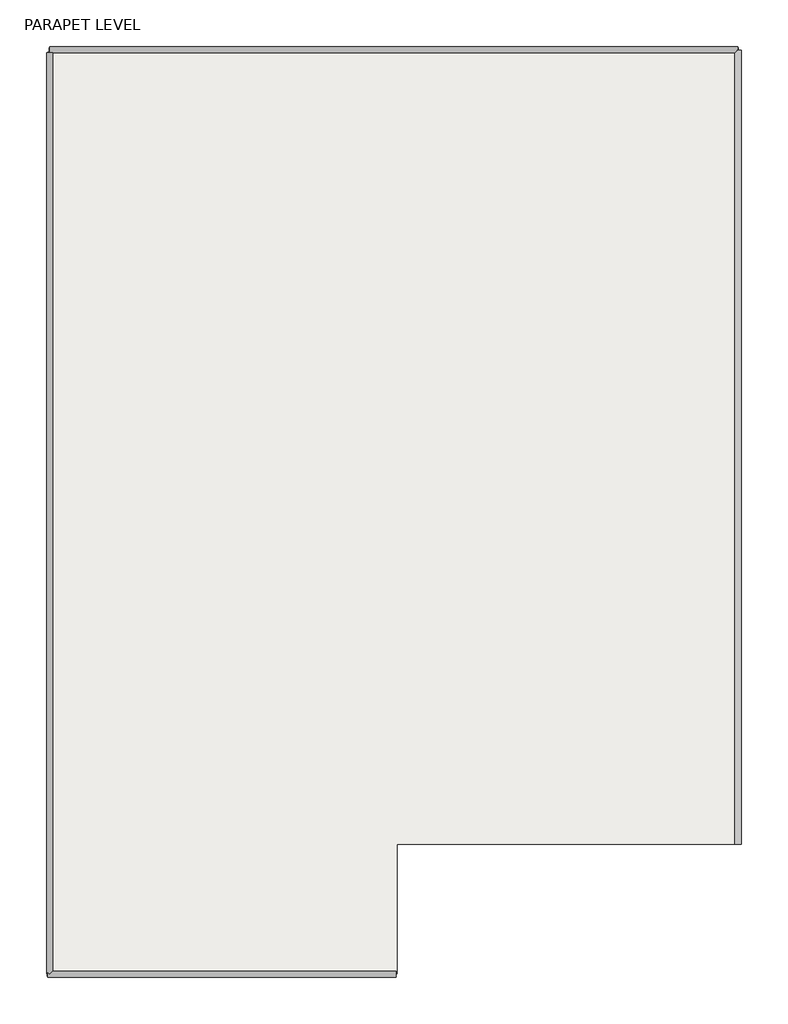
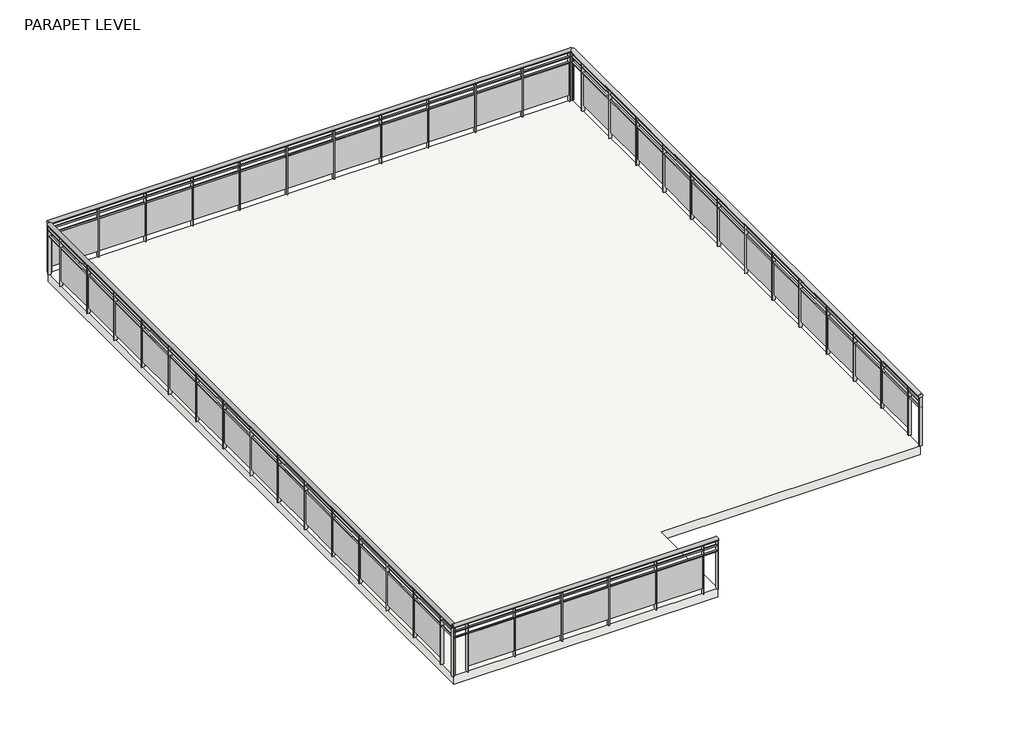
# One storey: 4 railings, 1 slab.
"""IFC4 building model written with IfcOpenShell, lengths in millimetres."""

from ifc_helpers import new_model, si_unit, point, frame, origin, place, context, project, spatial, polyline, ellipse_curve, trimmed, outline, extrude, element, save
from ifc_brep_helpers import plane_surface, extruded_surface, advanced_brep

model = new_model("IFC4")

# Units and contexts
model_context = context("Model", 3, world=origin())
ifc_project = project(units=[si_unit("LENGTHUNIT", "METRE", prefix="MILLI")], contexts=[model_context])

# Site, building, storey
site = spatial("IfcSite", under=ifc_project)
building = spatial("IfcBuilding", under=site)
storey = spatial("IfcBuildingStorey", under=building, Name="PARAPET LEVEL", Elevation=10546.08)

# Railings
placement = place(None, origin())
element("IfcRailing", 1, ObjectType="Glass_Panel-Bottom_Fill", at=placement, inside=storey, context=model_context, shape_type="SolidModel", body=[
    advanced_brep(
    [(-14979.3420435, 42.847874, 10681.6416), (-14979.3420435, -37.152126, 10681.6416), (-6089.3420435, 42.847874, 10681.6416), (-6089.3420435, -37.152126, 10681.6416)],
    [
        (0, 1, ellipse_curve(frame((-14979.3420435, 2.847874, 10681.6416), z_axis=(-1.0, 0.0, 0.0), x_axis=(0.0, -1.0, 0.0)), 40.0, 30.0)),
        (1, 0, ellipse_curve(frame((-14979.3420435, 2.847874, 10681.6416), z_axis=(-1.0, 0.0, 0.0), x_axis=(0.0, -1.0, 0.0)), 40.0, 30.0)),
        (2, 3, ellipse_curve(frame((-6089.3420435, 2.847874, 10681.6416), z_axis=(1.0, 0.0, 0.0), x_axis=(0.0, -1.0, 0.0)), 40.0, 30.0)),
        (3, 2, ellipse_curve(frame((-6089.3420435, 2.847874, 10681.6416), z_axis=(1.0, 0.0, 0.0), x_axis=(0.0, -1.0, 0.0)), 40.0, 30.0)),
        (0, 2),
        (3, 1),
    ],
    [
        plane_surface(frame((-14979.3420435, 2.847874, 10681.6416), z_axis=(-1.0, 0.0, 0.0), x_axis=(0.0, 1.0, 0.0))),
        plane_surface(frame((-6089.3420435, 2.847874, 10681.6416), z_axis=(1.0, 0.0, 0.0), x_axis=(0.0, 1.0, 0.0))),
        extruded_surface(trimmed(ellipse_curve(frame((-6089.3420435, 2.847874, 10681.6416), z_axis=(-1.0, 0.0, 0.0), x_axis=(0.0, -1.0, 0.0)), 40.0, 30.0), [point((-6089.3420435, 42.847874, 10681.6416))], [point((-6089.3420435, -37.152126, 10681.6416))], True, "CARTESIAN"), (-8890.0, 0.0, 0.0), 8890.0),
        extruded_surface(trimmed(ellipse_curve(frame((-6089.3420435, 2.847874, 10681.6416), z_axis=(-1.0, 0.0, 0.0), x_axis=(0.0, -1.0, 0.0)), 40.0, 30.0), [point((-6089.3420435, -37.152126, 10681.6416))], [point((-6089.3420435, 42.847874, 10681.6416))], True, "CARTESIAN"), (-8890.0, 0.0, 0.0), 8890.0),
    ],
    [
        (0, [[1, 2]]),
        (1, [[3, 4]]),
        (2, [[-1, 5, -4, 6]]),
        (3, [[-2, -6, -3, -5]]),
    ],
),
    extrude(outline(polyline([(-14979.3420435, -6.5428911), (-14979.3420435, 13.4571089), (-6089.3420435, 13.4571089), (-6089.3420435, -6.5428911), (-14979.3420435, -6.5428911)])), frame((0.0, 0.0, 10561.6416), z_axis=(0.0, 0.0, 1.0), x_axis=(1.0, 0.0, 0.0)), (0.0, 0.0, 1.0), 20.0),
    extrude(outline(polyline([(-14979.3420435, -6.5428911), (-14979.3420435, 13.4571089), (-6089.3420435, 13.4571089), (-6089.3420435, -6.5428911), (-14979.3420435, -6.5428911)])), frame((0.0, 0.0, 10461.6416), z_axis=(0.0, 0.0, 1.0), x_axis=(1.0, 0.0, 0.0)), (0.0, 0.0, 1.0), 20.0),
    extrude(outline(polyline([(-6140.3420435, 28.4571089), (-6128.3420435, 28.4571089), (-6128.3420435, -21.5428911), (-6140.3420435, -21.5428911), (-6140.3420435, 28.4571089)])), frame((0.0, 0.0, 9781.6416), z_axis=(0.0, 0.0, 1.0), x_axis=(1.0, 0.0, 0.0)), (0.0, 0.0, 1.0), 870.0),
    extrude(outline(polyline([(-6934.3420435, 1.7322988), (-6134.3420435, 1.7322988), (-6134.3420435, -3.2677012), (-6934.3420435, -3.2677012), (-6934.3420435, 1.7322988)])), frame((0.0, 0.0, 9881.6416), z_axis=(0.0, 0.0, 1.0), x_axis=(1.0, 0.0, 0.0)), (0.0, 0.0, 1.0), 580.0),
    extrude(outline(polyline([(-6940.3420435, 28.4571089), (-6928.3420435, 28.4571089), (-6928.3420435, -21.5428911), (-6940.3420435, -21.5428911), (-6940.3420435, 28.4571089)])), frame((0.0, 0.0, 9781.6416), z_axis=(0.0, 0.0, 1.0), x_axis=(1.0, 0.0, 0.0)), (0.0, 0.0, 1.0), 870.0),
    extrude(outline(polyline([(-7734.3420435, 1.7322988), (-6934.3420435, 1.7322988), (-6934.3420435, -3.2677012), (-7734.3420435, -3.2677012), (-7734.3420435, 1.7322988)])), frame((0.0, 0.0, 9881.6416), z_axis=(0.0, 0.0, 1.0), x_axis=(1.0, 0.0, 0.0)), (0.0, 0.0, 1.0), 580.0),
    extrude(outline(polyline([(-7740.3420435, 28.4571089), (-7728.3420435, 28.4571089), (-7728.3420435, -21.5428911), (-7740.3420435, -21.5428911), (-7740.3420435, 28.4571089)])), frame((0.0, 0.0, 9781.6416), z_axis=(0.0, 0.0, 1.0), x_axis=(1.0, 0.0, 0.0)), (0.0, 0.0, 1.0), 870.0),
    extrude(outline(polyline([(-8534.3420435, 1.7322988), (-7734.3420435, 1.7322988), (-7734.3420435, -3.2677012), (-8534.3420435, -3.2677012), (-8534.3420435, 1.7322988)])), frame((0.0, 0.0, 9881.6416), z_axis=(0.0, 0.0, 1.0), x_axis=(1.0, 0.0, 0.0)), (0.0, 0.0, 1.0), 580.0),
    extrude(outline(polyline([(-8540.3420435, 28.4571089), (-8528.3420435, 28.4571089), (-8528.3420435, -21.5428911), (-8540.3420435, -21.5428911), (-8540.3420435, 28.4571089)])), frame((0.0, 0.0, 9781.6416), z_axis=(0.0, 0.0, 1.0), x_axis=(1.0, 0.0, 0.0)), (0.0, 0.0, 1.0), 870.0),
    extrude(outline(polyline([(-9334.3420435, 1.7322988), (-8534.3420435, 1.7322988), (-8534.3420435, -3.2677012), (-9334.3420435, -3.2677012), (-9334.3420435, 1.7322988)])), frame((0.0, 0.0, 9881.6416), z_axis=(0.0, 0.0, 1.0), x_axis=(1.0, 0.0, 0.0)), (0.0, 0.0, 1.0), 580.0),
    extrude(outline(polyline([(-9340.3420435, 28.4571089), (-9328.3420435, 28.4571089), (-9328.3420435, -21.5428911), (-9340.3420435, -21.5428911), (-9340.3420435, 28.4571089)])), frame((0.0, 0.0, 9781.6416), z_axis=(0.0, 0.0, 1.0), x_axis=(1.0, 0.0, 0.0)), (0.0, 0.0, 1.0), 870.0),
    extrude(outline(polyline([(-10134.3420435, 1.7322988), (-9334.3420435, 1.7322988), (-9334.3420435, -3.2677012), (-10134.3420435, -3.2677012), (-10134.3420435, 1.7322988)])), frame((0.0, 0.0, 9881.6416), z_axis=(0.0, 0.0, 1.0), x_axis=(1.0, 0.0, 0.0)), (0.0, 0.0, 1.0), 580.0),
    extrude(outline(polyline([(-10140.3420435, 28.4571089), (-10128.3420435, 28.4571089), (-10128.3420435, -21.5428911), (-10140.3420435, -21.5428911), (-10140.3420435, 28.4571089)])), frame((0.0, 0.0, 9781.6416), z_axis=(0.0, 0.0, 1.0), x_axis=(1.0, 0.0, 0.0)), (0.0, 0.0, 1.0), 870.0),
    extrude(outline(polyline([(-10934.3420435, 1.7322988), (-10134.3420435, 1.7322988), (-10134.3420435, -3.2677012), (-10934.3420435, -3.2677012), (-10934.3420435, 1.7322988)])), frame((0.0, 0.0, 9881.6416), z_axis=(0.0, 0.0, 1.0), x_axis=(1.0, 0.0, 0.0)), (0.0, 0.0, 1.0), 580.0),
    extrude(outline(polyline([(-10940.3420435, 28.4571089), (-10928.3420435, 28.4571089), (-10928.3420435, -21.5428911), (-10940.3420435, -21.5428911), (-10940.3420435, 28.4571089)])), frame((0.0, 0.0, 9781.6416), z_axis=(0.0, 0.0, 1.0), x_axis=(1.0, 0.0, 0.0)), (0.0, 0.0, 1.0), 870.0),
    extrude(outline(polyline([(-11734.3420435, 1.7322988), (-10934.3420435, 1.7322988), (-10934.3420435, -3.2677012), (-11734.3420435, -3.2677012), (-11734.3420435, 1.7322988)])), frame((0.0, 0.0, 9881.6416), z_axis=(0.0, 0.0, 1.0), x_axis=(1.0, 0.0, 0.0)), (0.0, 0.0, 1.0), 580.0),
    extrude(outline(polyline([(-11740.3420435, 28.4571089), (-11728.3420435, 28.4571089), (-11728.3420435, -21.5428911), (-11740.3420435, -21.5428911), (-11740.3420435, 28.4571089)])), frame((0.0, 0.0, 9781.6416), z_axis=(0.0, 0.0, 1.0), x_axis=(1.0, 0.0, 0.0)), (0.0, 0.0, 1.0), 870.0),
    extrude(outline(polyline([(-12534.3420435, 1.7322988), (-11734.3420435, 1.7322988), (-11734.3420435, -3.2677012), (-12534.3420435, -3.2677012), (-12534.3420435, 1.7322988)])), frame((0.0, 0.0, 9881.6416), z_axis=(0.0, 0.0, 1.0), x_axis=(1.0, 0.0, 0.0)), (0.0, 0.0, 1.0), 580.0),
    extrude(outline(polyline([(-12540.3420435, 28.4571089), (-12528.3420435, 28.4571089), (-12528.3420435, -21.5428911), (-12540.3420435, -21.5428911), (-12540.3420435, 28.4571089)])), frame((0.0, 0.0, 9781.6416), z_axis=(0.0, 0.0, 1.0), x_axis=(1.0, 0.0, 0.0)), (0.0, 0.0, 1.0), 870.0),
    extrude(outline(polyline([(-13334.3420435, 1.7322988), (-12534.3420435, 1.7322988), (-12534.3420435, -3.2677012), (-13334.3420435, -3.2677012), (-13334.3420435, 1.7322988)])), frame((0.0, 0.0, 9881.6416), z_axis=(0.0, 0.0, 1.0), x_axis=(1.0, 0.0, 0.0)), (0.0, 0.0, 1.0), 580.0),
    extrude(outline(polyline([(-13340.3420435, 28.4571089), (-13328.3420435, 28.4571089), (-13328.3420435, -21.5428911), (-13340.3420435, -21.5428911), (-13340.3420435, 28.4571089)])), frame((0.0, 0.0, 9781.6416), z_axis=(0.0, 0.0, 1.0), x_axis=(1.0, 0.0, 0.0)), (0.0, 0.0, 1.0), 870.0),
    extrude(outline(polyline([(-14134.3420435, 1.7322988), (-13334.3420435, 1.7322988), (-13334.3420435, -3.2677012), (-14134.3420435, -3.2677012), (-14134.3420435, 1.7322988)])), frame((0.0, 0.0, 9881.6416), z_axis=(0.0, 0.0, 1.0), x_axis=(1.0, 0.0, 0.0)), (0.0, 0.0, 1.0), 580.0),
    extrude(outline(polyline([(-14140.3420435, 28.4571089), (-14128.3420435, 28.4571089), (-14128.3420435, -21.5428911), (-14140.3420435, -21.5428911), (-14140.3420435, 28.4571089)])), frame((0.0, 0.0, 9781.6416), z_axis=(0.0, 0.0, 1.0), x_axis=(1.0, 0.0, 0.0)), (0.0, 0.0, 1.0), 870.0),
    extrude(outline(polyline([(-14934.3420435, 1.7322988), (-14134.3420435, 1.7322988), (-14134.3420435, -3.2677012), (-14934.3420435, -3.2677012), (-14934.3420435, 1.7322988)])), frame((0.0, 0.0, 9881.6416), z_axis=(0.0, 0.0, 1.0), x_axis=(1.0, 0.0, 0.0)), (0.0, 0.0, 1.0), 580.0),
    extrude(outline(polyline([(-14940.3420435, 28.4571089), (-14928.3420435, 28.4571089), (-14928.3420435, -21.5428911), (-14940.3420435, -21.5428911), (-14940.3420435, 28.4571089)])), frame((0.0, 0.0, 9781.6416), z_axis=(0.0, 0.0, 1.0), x_axis=(1.0, 0.0, 0.0)), (0.0, 0.0, 1.0), 870.0),
    extrude(outline(polyline([(-6097.3420435, 28.4571089), (-6085.3420435, 28.4571089), (-6085.3420435, -21.5428911), (-6097.3420435, -21.5428911), (-6097.3420435, 28.4571089)])), frame((0.0, 0.0, 9781.6416), z_axis=(0.0, 0.0, 1.0), x_axis=(1.0, 0.0, 0.0)), (0.0, 0.0, 1.0), 870.0),
    extrude(outline(polyline([(-14983.3420435, 28.4571089), (-14971.3420435, 28.4571089), (-14971.3420435, -21.5428911), (-14983.3420435, -21.5428911), (-14983.3420435, 28.4571089)])), frame((0.0, 0.0, 9781.6416), z_axis=(0.0, 0.0, 1.0), x_axis=(1.0, 0.0, 0.0)), (0.0, 0.0, 1.0), 870.0),
])
element("IfcRailing", 2, ObjectType="Glass_Panel-Bottom_Fill", at=placement, inside=storey, context=model_context, shape_type="SolidModel", body=[
    advanced_brep(
    [(-14939.9512783, -37.152126, 10681.6416), (-15019.9512783, -37.152126, 10681.6416), (-14939.9512783, -11928.1928911, 10681.6416), (-15019.9512783, -11928.1928911, 10681.6416)],
    [
        (0, 1, ellipse_curve(frame((-14979.9512783, -37.152126, 10681.6416), z_axis=(0.0, 1.0, 0.0), x_axis=(-1.0, 0.0, 0.0)), 40.0, 30.0)),
        (1, 0, ellipse_curve(frame((-14979.9512783, -37.152126, 10681.6416), z_axis=(0.0, 1.0, 0.0), x_axis=(-1.0, 0.0, 0.0)), 40.0, 30.0)),
        (2, 3, ellipse_curve(frame((-14979.9512783, -11928.1928911, 10681.6416), z_axis=(0.0, -1.0, 0.0), x_axis=(-1.0, 0.0, 0.0)), 40.0, 30.0)),
        (3, 2, ellipse_curve(frame((-14979.9512783, -11928.1928911, 10681.6416), z_axis=(0.0, -1.0, 0.0), x_axis=(-1.0, 0.0, 0.0)), 40.0, 30.0)),
        (0, 2),
        (3, 1),
    ],
    [
        plane_surface(frame((-14979.9512783, -37.152126, 10681.6416), z_axis=(0.0, 1.0, 0.0), x_axis=(0.0, 0.0, -1.0))),
        plane_surface(frame((-14979.9512783, -11928.1928911, 10681.6416), z_axis=(0.0, -1.0, 0.0), x_axis=(0.0, 0.0, -1.0))),
        extruded_surface(trimmed(ellipse_curve(frame((-14979.9512783, -11928.1928911, 10681.6416), z_axis=(0.0, 1.0, 0.0), x_axis=(-1.0, 0.0, 0.0)), 40.0, 30.0), [point((-14939.9512783, -11928.1928911, 10681.6416))], [point((-15019.9512783, -11928.1928911, 10681.6416))], True, "CARTESIAN"), (0.0, 11891.040765099999, 0.0), 11891.040765099999),
        extruded_surface(trimmed(ellipse_curve(frame((-14979.9512783, -11928.1928911, 10681.6416), z_axis=(0.0, 1.0, 0.0), x_axis=(-1.0, 0.0, 0.0)), 40.0, 30.0), [point((-15019.9512783, -11928.1928911, 10681.6416))], [point((-14939.9512783, -11928.1928911, 10681.6416))], True, "CARTESIAN"), (0.0, 11891.040765099999, 0.0), 11891.040765099999),
    ],
    [
        (0, [[1, 2]]),
        (1, [[3, 4]]),
        (2, [[-1, 5, -4, 6]]),
        (3, [[-2, -6, -3, -5]]),
    ],
),
    extrude(outline(polyline([(-14989.3420435, -37.152126), (-14969.3420435, -37.152126), (-14969.3420435, -11928.1928911), (-14989.3420435, -11928.1928911), (-14989.3420435, -37.152126)])), frame((0.0, 0.0, 10561.6416), z_axis=(0.0, 0.0, 1.0), x_axis=(1.0, 0.0, 0.0)), (0.0, 0.0, 1.0), 20.0),
    extrude(outline(polyline([(-14989.3420435, -37.152126), (-14969.3420435, -37.152126), (-14969.3420435, -11928.1928911), (-14989.3420435, -11928.1928911), (-14989.3420435, -37.152126)])), frame((0.0, 0.0, 10461.6416), z_axis=(0.0, 0.0, 1.0), x_axis=(1.0, 0.0, 0.0)), (0.0, 0.0, 1.0), 20.0),
    extrude(outline(polyline([(-14954.3420435, -11576.6725086), (-14954.3420435, -11588.6725086), (-15004.3420435, -11588.6725086), (-15004.3420435, -11576.6725086), (-14954.3420435, -11576.6725086)])), frame((0.0, 0.0, 9781.6416), z_axis=(0.0, 0.0, 1.0), x_axis=(1.0, 0.0, 0.0)), (0.0, 0.0, 1.0), 870.0),
    extrude(outline(polyline([(-14981.0668536, -10782.6725086), (-14981.0668536, -11582.6725086), (-14986.0668536, -11582.6725086), (-14986.0668536, -10782.6725086), (-14981.0668536, -10782.6725086)])), frame((0.0, 0.0, 9881.6416), z_axis=(0.0, 0.0, 1.0), x_axis=(1.0, 0.0, 0.0)), (0.0, 0.0, 1.0), 580.0),
    extrude(outline(polyline([(-14954.3420435, -10776.6725086), (-14954.3420435, -10788.6725086), (-15004.3420435, -10788.6725086), (-15004.3420435, -10776.6725086), (-14954.3420435, -10776.6725086)])), frame((0.0, 0.0, 9781.6416), z_axis=(0.0, 0.0, 1.0), x_axis=(1.0, 0.0, 0.0)), (0.0, 0.0, 1.0), 870.0),
    extrude(outline(polyline([(-14981.0668536, -9982.6725086), (-14981.0668536, -10782.6725086), (-14986.0668536, -10782.6725086), (-14986.0668536, -9982.6725086), (-14981.0668536, -9982.6725086)])), frame((0.0, 0.0, 9881.6416), z_axis=(0.0, 0.0, 1.0), x_axis=(1.0, 0.0, 0.0)), (0.0, 0.0, 1.0), 580.0),
    extrude(outline(polyline([(-14954.3420435, -9976.6725086), (-14954.3420435, -9988.6725086), (-15004.3420435, -9988.6725086), (-15004.3420435, -9976.6725086), (-14954.3420435, -9976.6725086)])), frame((0.0, 0.0, 9781.6416), z_axis=(0.0, 0.0, 1.0), x_axis=(1.0, 0.0, 0.0)), (0.0, 0.0, 1.0), 870.0),
    extrude(outline(polyline([(-14981.0668536, -9182.6725086), (-14981.0668536, -9982.6725086), (-14986.0668536, -9982.6725086), (-14986.0668536, -9182.6725086), (-14981.0668536, -9182.6725086)])), frame((0.0, 0.0, 9881.6416), z_axis=(0.0, 0.0, 1.0), x_axis=(1.0, 0.0, 0.0)), (0.0, 0.0, 1.0), 580.0),
    extrude(outline(polyline([(-14954.3420435, -9176.6725086), (-14954.3420435, -9188.6725086), (-15004.3420435, -9188.6725086), (-15004.3420435, -9176.6725086), (-14954.3420435, -9176.6725086)])), frame((0.0, 0.0, 9781.6416), z_axis=(0.0, 0.0, 1.0), x_axis=(1.0, 0.0, 0.0)), (0.0, 0.0, 1.0), 870.0),
    extrude(outline(polyline([(-14981.0668536, -8382.6725086), (-14981.0668536, -9182.6725086), (-14986.0668536, -9182.6725086), (-14986.0668536, -8382.6725086), (-14981.0668536, -8382.6725086)])), frame((0.0, 0.0, 9881.6416), z_axis=(0.0, 0.0, 1.0), x_axis=(1.0, 0.0, 0.0)), (0.0, 0.0, 1.0), 580.0),
    extrude(outline(polyline([(-14954.3420435, -8376.6725086), (-14954.3420435, -8388.6725086), (-15004.3420435, -8388.6725086), (-15004.3420435, -8376.6725086), (-14954.3420435, -8376.6725086)])), frame((0.0, 0.0, 9781.6416), z_axis=(0.0, 0.0, 1.0), x_axis=(1.0, 0.0, 0.0)), (0.0, 0.0, 1.0), 870.0),
    extrude(outline(polyline([(-14981.0668536, -7582.6725086), (-14981.0668536, -8382.6725086), (-14986.0668536, -8382.6725086), (-14986.0668536, -7582.6725086), (-14981.0668536, -7582.6725086)])), frame((0.0, 0.0, 9881.6416), z_axis=(0.0, 0.0, 1.0), x_axis=(1.0, 0.0, 0.0)), (0.0, 0.0, 1.0), 580.0),
    extrude(outline(polyline([(-14954.3420435, -7576.6725086), (-14954.3420435, -7588.6725086), (-15004.3420435, -7588.6725086), (-15004.3420435, -7576.6725086), (-14954.3420435, -7576.6725086)])), frame((0.0, 0.0, 9781.6416), z_axis=(0.0, 0.0, 1.0), x_axis=(1.0, 0.0, 0.0)), (0.0, 0.0, 1.0), 870.0),
    extrude(outline(polyline([(-14981.0668536, -6782.6725086), (-14981.0668536, -7582.6725086), (-14986.0668536, -7582.6725086), (-14986.0668536, -6782.6725086), (-14981.0668536, -6782.6725086)])), frame((0.0, 0.0, 9881.6416), z_axis=(0.0, 0.0, 1.0), x_axis=(1.0, 0.0, 0.0)), (0.0, 0.0, 1.0), 580.0),
    extrude(outline(polyline([(-14954.3420435, -6776.6725086), (-14954.3420435, -6788.6725086), (-15004.3420435, -6788.6725086), (-15004.3420435, -6776.6725086), (-14954.3420435, -6776.6725086)])), frame((0.0, 0.0, 9781.6416), z_axis=(0.0, 0.0, 1.0), x_axis=(1.0, 0.0, 0.0)), (0.0, 0.0, 1.0), 870.0),
    extrude(outline(polyline([(-14981.0668536, -5982.6725086), (-14981.0668536, -6782.6725086), (-14986.0668536, -6782.6725086), (-14986.0668536, -5982.6725086), (-14981.0668536, -5982.6725086)])), frame((0.0, 0.0, 9881.6416), z_axis=(0.0, 0.0, 1.0), x_axis=(1.0, 0.0, 0.0)), (0.0, 0.0, 1.0), 580.0),
    extrude(outline(polyline([(-14954.3420435, -5976.6725086), (-14954.3420435, -5988.6725086), (-15004.3420435, -5988.6725086), (-15004.3420435, -5976.6725086), (-14954.3420435, -5976.6725086)])), frame((0.0, 0.0, 9781.6416), z_axis=(0.0, 0.0, 1.0), x_axis=(1.0, 0.0, 0.0)), (0.0, 0.0, 1.0), 870.0),
    extrude(outline(polyline([(-14981.0668536, -5182.6725086), (-14981.0668536, -5982.6725086), (-14986.0668536, -5982.6725086), (-14986.0668536, -5182.6725086), (-14981.0668536, -5182.6725086)])), frame((0.0, 0.0, 9881.6416), z_axis=(0.0, 0.0, 1.0), x_axis=(1.0, 0.0, 0.0)), (0.0, 0.0, 1.0), 580.0),
    extrude(outline(polyline([(-14954.3420435, -5176.6725086), (-14954.3420435, -5188.6725086), (-15004.3420435, -5188.6725086), (-15004.3420435, -5176.6725086), (-14954.3420435, -5176.6725086)])), frame((0.0, 0.0, 9781.6416), z_axis=(0.0, 0.0, 1.0), x_axis=(1.0, 0.0, 0.0)), (0.0, 0.0, 1.0), 870.0),
    extrude(outline(polyline([(-14981.0668536, -4382.6725086), (-14981.0668536, -5182.6725086), (-14986.0668536, -5182.6725086), (-14986.0668536, -4382.6725086), (-14981.0668536, -4382.6725086)])), frame((0.0, 0.0, 9881.6416), z_axis=(0.0, 0.0, 1.0), x_axis=(1.0, 0.0, 0.0)), (0.0, 0.0, 1.0), 580.0),
    extrude(outline(polyline([(-14954.3420435, -4376.6725086), (-14954.3420435, -4388.6725086), (-15004.3420435, -4388.6725086), (-15004.3420435, -4376.6725086), (-14954.3420435, -4376.6725086)])), frame((0.0, 0.0, 9781.6416), z_axis=(0.0, 0.0, 1.0), x_axis=(1.0, 0.0, 0.0)), (0.0, 0.0, 1.0), 870.0),
    extrude(outline(polyline([(-14981.0668536, -3582.6725086), (-14981.0668536, -4382.6725086), (-14986.0668536, -4382.6725086), (-14986.0668536, -3582.6725086), (-14981.0668536, -3582.6725086)])), frame((0.0, 0.0, 9881.6416), z_axis=(0.0, 0.0, 1.0), x_axis=(1.0, 0.0, 0.0)), (0.0, 0.0, 1.0), 580.0),
    extrude(outline(polyline([(-14954.3420435, -3576.6725086), (-14954.3420435, -3588.6725086), (-15004.3420435, -3588.6725086), (-15004.3420435, -3576.6725086), (-14954.3420435, -3576.6725086)])), frame((0.0, 0.0, 9781.6416), z_axis=(0.0, 0.0, 1.0), x_axis=(1.0, 0.0, 0.0)), (0.0, 0.0, 1.0), 870.0),
    extrude(outline(polyline([(-14981.0668536, -2782.6725086), (-14981.0668536, -3582.6725086), (-14986.0668536, -3582.6725086), (-14986.0668536, -2782.6725086), (-14981.0668536, -2782.6725086)])), frame((0.0, 0.0, 9881.6416), z_axis=(0.0, 0.0, 1.0), x_axis=(1.0, 0.0, 0.0)), (0.0, 0.0, 1.0), 580.0),
    extrude(outline(polyline([(-14954.3420435, -2776.6725086), (-14954.3420435, -2788.6725086), (-15004.3420435, -2788.6725086), (-15004.3420435, -2776.6725086), (-14954.3420435, -2776.6725086)])), frame((0.0, 0.0, 9781.6416), z_axis=(0.0, 0.0, 1.0), x_axis=(1.0, 0.0, 0.0)), (0.0, 0.0, 1.0), 870.0),
    extrude(outline(polyline([(-14981.0668536, -1982.6725086), (-14981.0668536, -2782.6725086), (-14986.0668536, -2782.6725086), (-14986.0668536, -1982.6725086), (-14981.0668536, -1982.6725086)])), frame((0.0, 0.0, 9881.6416), z_axis=(0.0, 0.0, 1.0), x_axis=(1.0, 0.0, 0.0)), (0.0, 0.0, 1.0), 580.0),
    extrude(outline(polyline([(-14954.3420435, -1976.6725086), (-14954.3420435, -1988.6725086), (-15004.3420435, -1988.6725086), (-15004.3420435, -1976.6725086), (-14954.3420435, -1976.6725086)])), frame((0.0, 0.0, 9781.6416), z_axis=(0.0, 0.0, 1.0), x_axis=(1.0, 0.0, 0.0)), (0.0, 0.0, 1.0), 870.0),
    extrude(outline(polyline([(-14981.0668536, -1182.6725086), (-14981.0668536, -1982.6725086), (-14986.0668536, -1982.6725086), (-14986.0668536, -1182.6725086), (-14981.0668536, -1182.6725086)])), frame((0.0, 0.0, 9881.6416), z_axis=(0.0, 0.0, 1.0), x_axis=(1.0, 0.0, 0.0)), (0.0, 0.0, 1.0), 580.0),
    extrude(outline(polyline([(-14954.3420435, -1176.6725086), (-14954.3420435, -1188.6725086), (-15004.3420435, -1188.6725086), (-15004.3420435, -1176.6725086), (-14954.3420435, -1176.6725086)])), frame((0.0, 0.0, 9781.6416), z_axis=(0.0, 0.0, 1.0), x_axis=(1.0, 0.0, 0.0)), (0.0, 0.0, 1.0), 870.0),
    extrude(outline(polyline([(-14981.0668536, -382.6725086), (-14981.0668536, -1182.6725086), (-14986.0668536, -1182.6725086), (-14986.0668536, -382.6725086), (-14981.0668536, -382.6725086)])), frame((0.0, 0.0, 9881.6416), z_axis=(0.0, 0.0, 1.0), x_axis=(1.0, 0.0, 0.0)), (0.0, 0.0, 1.0), 580.0),
    extrude(outline(polyline([(-14954.3420435, -376.6725086), (-14954.3420435, -388.6725086), (-15004.3420435, -388.6725086), (-15004.3420435, -376.6725086), (-14954.3420435, -376.6725086)])), frame((0.0, 0.0, 9781.6416), z_axis=(0.0, 0.0, 1.0), x_axis=(1.0, 0.0, 0.0)), (0.0, 0.0, 1.0), 870.0),
    extrude(outline(polyline([(-14954.3420435, -11920.1928911), (-14954.3420435, -11932.1928911), (-15004.3420435, -11932.1928911), (-15004.3420435, -11920.1928911), (-14954.3420435, -11920.1928911)])), frame((0.0, 0.0, 9781.6416), z_axis=(0.0, 0.0, 1.0), x_axis=(1.0, 0.0, 0.0)), (0.0, 0.0, 1.0), 870.0),
    extrude(outline(polyline([(-14954.3420435, -33.152126), (-14954.3420435, -45.152126), (-15004.3420435, -45.152126), (-15004.3420435, -33.152126), (-14954.3420435, -33.152126)])), frame((0.0, 0.0, 9781.6416), z_axis=(0.0, 0.0, 1.0), x_axis=(1.0, 0.0, 0.0)), (0.0, 0.0, 1.0), 870.0),
])
element("IfcRailing", 3, ObjectType="Glass_Panel-Bottom_Fill", at=placement, inside=storey, context=model_context, shape_type="SolidModel", body=[
    advanced_brep(
    [(-15004.3420435, -11892.802126, 10681.6416), (-15004.3420435, -11972.802126, 10681.6416), (-10508.5420435, -11892.802126, 10681.6416), (-10508.5420435, -11972.802126, 10681.6416)],
    [
        (0, 1, ellipse_curve(frame((-15004.3420435, -11932.802126, 10681.6416), z_axis=(-1.0, 0.0, 0.0), x_axis=(0.0, -1.0, 0.0)), 40.0, 30.0)),
        (1, 0, ellipse_curve(frame((-15004.3420435, -11932.802126, 10681.6416), z_axis=(-1.0, 0.0, 0.0), x_axis=(0.0, -1.0, 0.0)), 40.0, 30.0)),
        (2, 3, ellipse_curve(frame((-10508.5420435, -11932.802126, 10681.6416), z_axis=(1.0, 0.0, 0.0), x_axis=(0.0, -1.0, 0.0)), 40.0, 30.0)),
        (3, 2, ellipse_curve(frame((-10508.5420435, -11932.802126, 10681.6416), z_axis=(1.0, 0.0, 0.0), x_axis=(0.0, -1.0, 0.0)), 40.0, 30.0)),
        (0, 2),
        (3, 1),
    ],
    [
        plane_surface(frame((-15004.3420435, -11932.802126, 10681.6416), z_axis=(-1.0, 0.0, 0.0), x_axis=(0.0, 1.0, 0.0))),
        plane_surface(frame((-10508.5420435, -11932.802126, 10681.6416), z_axis=(1.0, 0.0, 0.0), x_axis=(0.0, 1.0, 0.0))),
        extruded_surface(trimmed(ellipse_curve(frame((-10508.5420435, -11932.802126, 10681.6416), z_axis=(-1.0, 0.0, 0.0), x_axis=(0.0, -1.0, 0.0)), 40.0, 30.0), [point((-10508.5420435, -11892.802126, 10681.6416))], [point((-10508.5420435, -11972.802126, 10681.6416))], True, "CARTESIAN"), (-4495.800000000001, 0.0, 0.0), 4495.800000000001),
        extruded_surface(trimmed(ellipse_curve(frame((-10508.5420435, -11932.802126, 10681.6416), z_axis=(-1.0, 0.0, 0.0), x_axis=(0.0, -1.0, 0.0)), 40.0, 30.0), [point((-10508.5420435, -11972.802126, 10681.6416))], [point((-10508.5420435, -11892.802126, 10681.6416))], True, "CARTESIAN"), (-4495.800000000001, 0.0, 0.0), 4495.800000000001),
    ],
    [
        (0, [[1, 2]]),
        (1, [[3, 4]]),
        (2, [[-1, 5, -4, 6]]),
        (3, [[-2, -6, -3, -5]]),
    ],
),
    extrude(outline(polyline([(-15004.3420435, -11942.1928911), (-15004.3420435, -11922.1928911), (-10508.5420435, -11922.1928911), (-10508.5420435, -11942.1928911), (-15004.3420435, -11942.1928911)])), frame((0.0, 0.0, 10561.6416), z_axis=(0.0, 0.0, 1.0), x_axis=(1.0, 0.0, 0.0)), (0.0, 0.0, 1.0), 20.0),
    extrude(outline(polyline([(-15004.3420435, -11942.1928911), (-15004.3420435, -11922.1928911), (-10508.5420435, -11922.1928911), (-10508.5420435, -11942.1928911), (-15004.3420435, -11942.1928911)])), frame((0.0, 0.0, 10461.6416), z_axis=(0.0, 0.0, 1.0), x_axis=(1.0, 0.0, 0.0)), (0.0, 0.0, 1.0), 20.0),
    extrude(outline(polyline([(-10762.4420435, -11907.1928911), (-10750.4420435, -11907.1928911), (-10750.4420435, -11957.1928911), (-10762.4420435, -11957.1928911), (-10762.4420435, -11907.1928911)])), frame((0.0, 0.0, 9781.6416), z_axis=(0.0, 0.0, 1.0), x_axis=(1.0, 0.0, 0.0)), (0.0, 0.0, 1.0), 870.0),
    extrude(outline(polyline([(-11556.4420435, -11933.9177012), (-10756.4420435, -11933.9177012), (-10756.4420435, -11938.9177012), (-11556.4420435, -11938.9177012), (-11556.4420435, -11933.9177012)])), frame((0.0, 0.0, 9881.6416), z_axis=(0.0, 0.0, 1.0), x_axis=(1.0, 0.0, 0.0)), (0.0, 0.0, 1.0), 580.0),
    extrude(outline(polyline([(-11562.4420435, -11907.1928911), (-11550.4420435, -11907.1928911), (-11550.4420435, -11957.1928911), (-11562.4420435, -11957.1928911), (-11562.4420435, -11907.1928911)])), frame((0.0, 0.0, 9781.6416), z_axis=(0.0, 0.0, 1.0), x_axis=(1.0, 0.0, 0.0)), (0.0, 0.0, 1.0), 870.0),
    extrude(outline(polyline([(-12356.4420435, -11933.9177012), (-11556.4420435, -11933.9177012), (-11556.4420435, -11938.9177012), (-12356.4420435, -11938.9177012), (-12356.4420435, -11933.9177012)])), frame((0.0, 0.0, 9881.6416), z_axis=(0.0, 0.0, 1.0), x_axis=(1.0, 0.0, 0.0)), (0.0, 0.0, 1.0), 580.0),
    extrude(outline(polyline([(-12362.4420435, -11907.1928911), (-12350.4420435, -11907.1928911), (-12350.4420435, -11957.1928911), (-12362.4420435, -11957.1928911), (-12362.4420435, -11907.1928911)])), frame((0.0, 0.0, 9781.6416), z_axis=(0.0, 0.0, 1.0), x_axis=(1.0, 0.0, 0.0)), (0.0, 0.0, 1.0), 870.0),
    extrude(outline(polyline([(-13156.4420435, -11933.9177012), (-12356.4420435, -11933.9177012), (-12356.4420435, -11938.9177012), (-13156.4420435, -11938.9177012), (-13156.4420435, -11933.9177012)])), frame((0.0, 0.0, 9881.6416), z_axis=(0.0, 0.0, 1.0), x_axis=(1.0, 0.0, 0.0)), (0.0, 0.0, 1.0), 580.0),
    extrude(outline(polyline([(-13162.4420435, -11907.1928911), (-13150.4420435, -11907.1928911), (-13150.4420435, -11957.1928911), (-13162.4420435, -11957.1928911), (-13162.4420435, -11907.1928911)])), frame((0.0, 0.0, 9781.6416), z_axis=(0.0, 0.0, 1.0), x_axis=(1.0, 0.0, 0.0)), (0.0, 0.0, 1.0), 870.0),
    extrude(outline(polyline([(-13956.4420435, -11933.9177012), (-13156.4420435, -11933.9177012), (-13156.4420435, -11938.9177012), (-13956.4420435, -11938.9177012), (-13956.4420435, -11933.9177012)])), frame((0.0, 0.0, 9881.6416), z_axis=(0.0, 0.0, 1.0), x_axis=(1.0, 0.0, 0.0)), (0.0, 0.0, 1.0), 580.0),
    extrude(outline(polyline([(-13962.4420435, -11907.1928911), (-13950.4420435, -11907.1928911), (-13950.4420435, -11957.1928911), (-13962.4420435, -11957.1928911), (-13962.4420435, -11907.1928911)])), frame((0.0, 0.0, 9781.6416), z_axis=(0.0, 0.0, 1.0), x_axis=(1.0, 0.0, 0.0)), (0.0, 0.0, 1.0), 870.0),
    extrude(outline(polyline([(-14756.4420435, -11933.9177012), (-13956.4420435, -11933.9177012), (-13956.4420435, -11938.9177012), (-14756.4420435, -11938.9177012), (-14756.4420435, -11933.9177012)])), frame((0.0, 0.0, 9881.6416), z_axis=(0.0, 0.0, 1.0), x_axis=(1.0, 0.0, 0.0)), (0.0, 0.0, 1.0), 580.0),
    extrude(outline(polyline([(-14762.4420435, -11907.1928911), (-14750.4420435, -11907.1928911), (-14750.4420435, -11957.1928911), (-14762.4420435, -11957.1928911), (-14762.4420435, -11907.1928911)])), frame((0.0, 0.0, 9781.6416), z_axis=(0.0, 0.0, 1.0), x_axis=(1.0, 0.0, 0.0)), (0.0, 0.0, 1.0), 870.0),
    extrude(outline(polyline([(-10516.5420435, -11907.1928911), (-10504.5420435, -11907.1928911), (-10504.5420435, -11957.1928911), (-10516.5420435, -11957.1928911), (-10516.5420435, -11907.1928911)])), frame((0.0, 0.0, 9781.6416), z_axis=(0.0, 0.0, 1.0), x_axis=(1.0, 0.0, 0.0)), (0.0, 0.0, 1.0), 870.0),
    extrude(outline(polyline([(-15008.3420435, -11907.1928911), (-14996.3420435, -11907.1928911), (-14996.3420435, -11957.1928911), (-15008.3420435, -11957.1928911), (-15008.3420435, -11907.1928911)])), frame((0.0, 0.0, 9781.6416), z_axis=(0.0, 0.0, 1.0), x_axis=(1.0, 0.0, 0.0)), (0.0, 0.0, 1.0), 870.0),
])
element("IfcRailing", 4, ObjectType="Glass_Panel-Bottom_Fill", at=placement, inside=storey, context=model_context, shape_type="SolidModel", body=[
    advanced_brep(
    [(-6128.7328087, -10251.7928911, 10681.6416), (-6048.7328087, -10251.7928911, 10681.6416), (-6128.7328087, -6.5428911, 10681.6416), (-6048.7328087, -6.5428911, 10681.6416)],
    [
        (0, 1, ellipse_curve(frame((-6088.7328087, -10251.7928911, 10681.6416), z_axis=(0.0, -1.0, 0.0), x_axis=(1.0, 0.0, 0.0)), 40.0, 30.0)),
        (1, 0, ellipse_curve(frame((-6088.7328087, -10251.7928911, 10681.6416), z_axis=(0.0, -1.0, 0.0), x_axis=(1.0, 0.0, 0.0)), 40.0, 30.0)),
        (2, 3, ellipse_curve(frame((-6088.7328087, -6.5428911, 10681.6416), z_axis=(0.0, 1.0, 0.0), x_axis=(1.0, 0.0, 0.0)), 40.0, 30.0)),
        (3, 2, ellipse_curve(frame((-6088.7328087, -6.5428911, 10681.6416), z_axis=(0.0, 1.0, 0.0), x_axis=(1.0, 0.0, 0.0)), 40.0, 30.0)),
        (0, 2),
        (3, 1),
    ],
    [
        plane_surface(frame((-6088.7328087, -10251.7928911, 10681.6416), z_axis=(0.0, -1.0, 0.0), x_axis=(0.0, 0.0, 1.0))),
        plane_surface(frame((-6088.7328087, -6.5428911, 10681.6416), z_axis=(0.0, 1.0, 0.0), x_axis=(0.0, 0.0, 1.0))),
        extruded_surface(trimmed(ellipse_curve(frame((-6088.7328087, -6.5428911, 10681.6416), z_axis=(0.0, -1.0, 0.0), x_axis=(1.0, 0.0, 0.0)), 40.0, 30.0), [point((-6128.7328087, -6.5428911, 10681.6416))], [point((-6048.7328087, -6.5428911, 10681.6416))], True, "CARTESIAN"), (0.0, -10245.25, 0.0), 10245.25),
        extruded_surface(trimmed(ellipse_curve(frame((-6088.7328087, -6.5428911, 10681.6416), z_axis=(0.0, -1.0, 0.0), x_axis=(1.0, 0.0, 0.0)), 40.0, 30.0), [point((-6048.7328087, -6.5428911, 10681.6416))], [point((-6128.7328087, -6.5428911, 10681.6416))], True, "CARTESIAN"), (0.0, -10245.25, 0.0), 10245.25),
    ],
    [
        (0, [[1, 2]]),
        (1, [[3, 4]]),
        (2, [[-1, 5, -4, 6]]),
        (3, [[-2, -6, -3, -5]]),
    ],
),
    extrude(outline(polyline([(-6079.3420435, -10251.7928911), (-6099.3420435, -10251.7928911), (-6099.3420435, -6.5428911), (-6079.3420435, -6.5428911), (-6079.3420435, -10251.7928911)])), frame((0.0, 0.0, 10561.6416), z_axis=(0.0, 0.0, 1.0), x_axis=(1.0, 0.0, 0.0)), (0.0, 0.0, 1.0), 20.0),
    extrude(outline(polyline([(-6079.3420435, -10251.7928911), (-6099.3420435, -10251.7928911), (-6099.3420435, -6.5428911), (-6079.3420435, -6.5428911), (-6079.3420435, -10251.7928911)])), frame((0.0, 0.0, 10461.6416), z_axis=(0.0, 0.0, 1.0), x_axis=(1.0, 0.0, 0.0)), (0.0, 0.0, 1.0), 20.0),
    extrude(outline(polyline([(-6114.3420435, -335.1678911), (-6114.3420435, -323.1678911), (-6064.3420435, -323.1678911), (-6064.3420435, -335.1678911), (-6114.3420435, -335.1678911)])), frame((0.0, 0.0, 9781.6416), z_axis=(0.0, 0.0, 1.0), x_axis=(1.0, 0.0, 0.0)), (0.0, 0.0, 1.0), 870.0),
    extrude(outline(polyline([(-6087.6172334, -1129.1678911), (-6087.6172334, -329.1678911), (-6082.6172334, -329.1678911), (-6082.6172334, -1129.1678911), (-6087.6172334, -1129.1678911)])), frame((0.0, 0.0, 9881.6416), z_axis=(0.0, 0.0, 1.0), x_axis=(1.0, 0.0, 0.0)), (0.0, 0.0, 1.0), 580.0),
    extrude(outline(polyline([(-6114.3420435, -1135.1678911), (-6114.3420435, -1123.1678911), (-6064.3420435, -1123.1678911), (-6064.3420435, -1135.1678911), (-6114.3420435, -1135.1678911)])), frame((0.0, 0.0, 9781.6416), z_axis=(0.0, 0.0, 1.0), x_axis=(1.0, 0.0, 0.0)), (0.0, 0.0, 1.0), 870.0),
    extrude(outline(polyline([(-6087.6172334, -1929.1678911), (-6087.6172334, -1129.1678911), (-6082.6172334, -1129.1678911), (-6082.6172334, -1929.1678911), (-6087.6172334, -1929.1678911)])), frame((0.0, 0.0, 9881.6416), z_axis=(0.0, 0.0, 1.0), x_axis=(1.0, 0.0, 0.0)), (0.0, 0.0, 1.0), 580.0),
    extrude(outline(polyline([(-6114.3420435, -1935.1678911), (-6114.3420435, -1923.1678911), (-6064.3420435, -1923.1678911), (-6064.3420435, -1935.1678911), (-6114.3420435, -1935.1678911)])), frame((0.0, 0.0, 9781.6416), z_axis=(0.0, 0.0, 1.0), x_axis=(1.0, 0.0, 0.0)), (0.0, 0.0, 1.0), 870.0),
    extrude(outline(polyline([(-6087.6172334, -2729.1678911), (-6087.6172334, -1929.1678911), (-6082.6172334, -1929.1678911), (-6082.6172334, -2729.1678911), (-6087.6172334, -2729.1678911)])), frame((0.0, 0.0, 9881.6416), z_axis=(0.0, 0.0, 1.0), x_axis=(1.0, 0.0, 0.0)), (0.0, 0.0, 1.0), 580.0),
    extrude(outline(polyline([(-6114.3420435, -2735.1678911), (-6114.3420435, -2723.1678911), (-6064.3420435, -2723.1678911), (-6064.3420435, -2735.1678911), (-6114.3420435, -2735.1678911)])), frame((0.0, 0.0, 9781.6416), z_axis=(0.0, 0.0, 1.0), x_axis=(1.0, 0.0, 0.0)), (0.0, 0.0, 1.0), 870.0),
    extrude(outline(polyline([(-6087.6172334, -3529.1678911), (-6087.6172334, -2729.1678911), (-6082.6172334, -2729.1678911), (-6082.6172334, -3529.1678911), (-6087.6172334, -3529.1678911)])), frame((0.0, 0.0, 9881.6416), z_axis=(0.0, 0.0, 1.0), x_axis=(1.0, 0.0, 0.0)), (0.0, 0.0, 1.0), 580.0),
    extrude(outline(polyline([(-6114.3420435, -3535.1678911), (-6114.3420435, -3523.1678911), (-6064.3420435, -3523.1678911), (-6064.3420435, -3535.1678911), (-6114.3420435, -3535.1678911)])), frame((0.0, 0.0, 9781.6416), z_axis=(0.0, 0.0, 1.0), x_axis=(1.0, 0.0, 0.0)), (0.0, 0.0, 1.0), 870.0),
    extrude(outline(polyline([(-6087.6172334, -4329.1678911), (-6087.6172334, -3529.1678911), (-6082.6172334, -3529.1678911), (-6082.6172334, -4329.1678911), (-6087.6172334, -4329.1678911)])), frame((0.0, 0.0, 9881.6416), z_axis=(0.0, 0.0, 1.0), x_axis=(1.0, 0.0, 0.0)), (0.0, 0.0, 1.0), 580.0),
    extrude(outline(polyline([(-6114.3420435, -4335.1678911), (-6114.3420435, -4323.1678911), (-6064.3420435, -4323.1678911), (-6064.3420435, -4335.1678911), (-6114.3420435, -4335.1678911)])), frame((0.0, 0.0, 9781.6416), z_axis=(0.0, 0.0, 1.0), x_axis=(1.0, 0.0, 0.0)), (0.0, 0.0, 1.0), 870.0),
    extrude(outline(polyline([(-6087.6172334, -5129.1678911), (-6087.6172334, -4329.1678911), (-6082.6172334, -4329.1678911), (-6082.6172334, -5129.1678911), (-6087.6172334, -5129.1678911)])), frame((0.0, 0.0, 9881.6416), z_axis=(0.0, 0.0, 1.0), x_axis=(1.0, 0.0, 0.0)), (0.0, 0.0, 1.0), 580.0),
    extrude(outline(polyline([(-6114.3420435, -5135.1678911), (-6114.3420435, -5123.1678911), (-6064.3420435, -5123.1678911), (-6064.3420435, -5135.1678911), (-6114.3420435, -5135.1678911)])), frame((0.0, 0.0, 9781.6416), z_axis=(0.0, 0.0, 1.0), x_axis=(1.0, 0.0, 0.0)), (0.0, 0.0, 1.0), 870.0),
    extrude(outline(polyline([(-6087.6172334, -5929.1678911), (-6087.6172334, -5129.1678911), (-6082.6172334, -5129.1678911), (-6082.6172334, -5929.1678911), (-6087.6172334, -5929.1678911)])), frame((0.0, 0.0, 9881.6416), z_axis=(0.0, 0.0, 1.0), x_axis=(1.0, 0.0, 0.0)), (0.0, 0.0, 1.0), 580.0),
    extrude(outline(polyline([(-6114.3420435, -5935.1678911), (-6114.3420435, -5923.1678911), (-6064.3420435, -5923.1678911), (-6064.3420435, -5935.1678911), (-6114.3420435, -5935.1678911)])), frame((0.0, 0.0, 9781.6416), z_axis=(0.0, 0.0, 1.0), x_axis=(1.0, 0.0, 0.0)), (0.0, 0.0, 1.0), 870.0),
    extrude(outline(polyline([(-6087.6172334, -6729.1678911), (-6087.6172334, -5929.1678911), (-6082.6172334, -5929.1678911), (-6082.6172334, -6729.1678911), (-6087.6172334, -6729.1678911)])), frame((0.0, 0.0, 9881.6416), z_axis=(0.0, 0.0, 1.0), x_axis=(1.0, 0.0, 0.0)), (0.0, 0.0, 1.0), 580.0),
    extrude(outline(polyline([(-6114.3420435, -6735.1678911), (-6114.3420435, -6723.1678911), (-6064.3420435, -6723.1678911), (-6064.3420435, -6735.1678911), (-6114.3420435, -6735.1678911)])), frame((0.0, 0.0, 9781.6416), z_axis=(0.0, 0.0, 1.0), x_axis=(1.0, 0.0, 0.0)), (0.0, 0.0, 1.0), 870.0),
    extrude(outline(polyline([(-6087.6172334, -7529.1678911), (-6087.6172334, -6729.1678911), (-6082.6172334, -6729.1678911), (-6082.6172334, -7529.1678911), (-6087.6172334, -7529.1678911)])), frame((0.0, 0.0, 9881.6416), z_axis=(0.0, 0.0, 1.0), x_axis=(1.0, 0.0, 0.0)), (0.0, 0.0, 1.0), 580.0),
    extrude(outline(polyline([(-6114.3420435, -7535.1678911), (-6114.3420435, -7523.1678911), (-6064.3420435, -7523.1678911), (-6064.3420435, -7535.1678911), (-6114.3420435, -7535.1678911)])), frame((0.0, 0.0, 9781.6416), z_axis=(0.0, 0.0, 1.0), x_axis=(1.0, 0.0, 0.0)), (0.0, 0.0, 1.0), 870.0),
    extrude(outline(polyline([(-6087.6172334, -8329.1678911), (-6087.6172334, -7529.1678911), (-6082.6172334, -7529.1678911), (-6082.6172334, -8329.1678911), (-6087.6172334, -8329.1678911)])), frame((0.0, 0.0, 9881.6416), z_axis=(0.0, 0.0, 1.0), x_axis=(1.0, 0.0, 0.0)), (0.0, 0.0, 1.0), 580.0),
    extrude(outline(polyline([(-6114.3420435, -8335.1678911), (-6114.3420435, -8323.1678911), (-6064.3420435, -8323.1678911), (-6064.3420435, -8335.1678911), (-6114.3420435, -8335.1678911)])), frame((0.0, 0.0, 9781.6416), z_axis=(0.0, 0.0, 1.0), x_axis=(1.0, 0.0, 0.0)), (0.0, 0.0, 1.0), 870.0),
    extrude(outline(polyline([(-6087.6172334, -9129.1678911), (-6087.6172334, -8329.1678911), (-6082.6172334, -8329.1678911), (-6082.6172334, -9129.1678911), (-6087.6172334, -9129.1678911)])), frame((0.0, 0.0, 9881.6416), z_axis=(0.0, 0.0, 1.0), x_axis=(1.0, 0.0, 0.0)), (0.0, 0.0, 1.0), 580.0),
    extrude(outline(polyline([(-6114.3420435, -9135.1678911), (-6114.3420435, -9123.1678911), (-6064.3420435, -9123.1678911), (-6064.3420435, -9135.1678911), (-6114.3420435, -9135.1678911)])), frame((0.0, 0.0, 9781.6416), z_axis=(0.0, 0.0, 1.0), x_axis=(1.0, 0.0, 0.0)), (0.0, 0.0, 1.0), 870.0),
    extrude(outline(polyline([(-6087.6172334, -9929.1678911), (-6087.6172334, -9129.1678911), (-6082.6172334, -9129.1678911), (-6082.6172334, -9929.1678911), (-6087.6172334, -9929.1678911)])), frame((0.0, 0.0, 9881.6416), z_axis=(0.0, 0.0, 1.0), x_axis=(1.0, 0.0, 0.0)), (0.0, 0.0, 1.0), 580.0),
    extrude(outline(polyline([(-6114.3420435, -9935.1678911), (-6114.3420435, -9923.1678911), (-6064.3420435, -9923.1678911), (-6064.3420435, -9935.1678911), (-6114.3420435, -9935.1678911)])), frame((0.0, 0.0, 9781.6416), z_axis=(0.0, 0.0, 1.0), x_axis=(1.0, 0.0, 0.0)), (0.0, 0.0, 1.0), 870.0),
    extrude(outline(polyline([(-6114.3420435, -14.5428911), (-6114.3420435, -2.5428911), (-6064.3420435, -2.5428911), (-6064.3420435, -14.5428911), (-6114.3420435, -14.5428911)])), frame((0.0, 0.0, 9781.6416), z_axis=(0.0, 0.0, 1.0), x_axis=(1.0, 0.0, 0.0)), (0.0, 0.0, 1.0), 870.0),
    extrude(outline(polyline([(-6114.3420435, -10255.7928911), (-6114.3420435, -10243.7928911), (-6064.3420435, -10243.7928911), (-6064.3420435, -10255.7928911), (-6114.3420435, -10255.7928911)])), frame((0.0, 0.0, 9781.6416), z_axis=(0.0, 0.0, 1.0), x_axis=(1.0, 0.0, 0.0)), (0.0, 0.0, 1.0), 870.0),
])

# Slab
element("IfcSlab", 5, ObjectType="OUTER FLOORING", at=placement, inside=storey, context=model_context, shape_type="SweptSolid", body=[
    extrude(outline(polyline([(-6089.3420435, 3.4571089), (-6089.3420435, -10251.7928911), (-10495.9340108, -10251.7928911), (-10495.9340108, -11928.1928911), (-14979.3420435, -11928.1928911), (-14979.3420435, 3.4571089), (-6089.3420435, 3.4571089)])), frame((0.0, 0.0, 9631.68), z_axis=(0.0, 0.0, 1.0), x_axis=(1.0, 0.0, 0.0)), (0.0, 0.0, 1.0), 149.9616),
])

save(model, "model.ifc")

# Revit data of these elements
# Type "Glass_Panel-Bottom_Fill"
#   built-in parameter 1008612 = 0.019685 (stored number, unit not read)
#   built-in parameter 1008611 = 0.019685 (stored number, unit not read)
#   built-in parameter 1008609 = 0.902231 (stored number, unit not read)
#   built-in parameter 1008604 = 0.19685 (stored number, unit not read)
#   built-in parameter 1008603 = 0.164042 (stored number, unit not read)
#   Railing Height = 2.952756 ft
#   built-in parameter 1008630 = 2
#   built-in parameter 1008610 = 2
# Type "OUTER FLOORING"
#   Function = 0
#   Layers, outside or top first: 0.072 ft "Concrete Masonry Units _High Density" (function 5); 0.42 ft "Structure, Timber Joist/Rafter Layer" (function 1)
# Elements 1, 2, 3, 4 (IfcRailing, "Glass_Panel-Bottom_Fill")
#   built-in parameter 1008621 = -2.508 (stored number, unit not read)
#   Phase Created = New Construction
#   Materials on its faces: "Metal - Stainless Steel,Polished", "Glass"
# Element 5 (IfcSlab, "OUTER FLOORING")
#   Height Offset From Level = -2.508 ft
#   Phase Created = New Construction
#   Materials on its faces: "Structure, Timber Joist/Rafter Layer", "Concrete Masonry Units _High Density"
# Materials
#   "Concrete Masonry Units _High Density": class "Masonry", colour RGB 181 181 181, transparency 0, Description = "Concrete masonry units", Cost = 0
#   "Structure, Timber Joist/Rafter Layer": class "Wood", colour RGB 127 127 127, transparency 0, Description = "Timber framing, thermal airspace", Cost = 0
#   "Metal - Stainless Steel,Polished": class "Metal", colour RGB 236 239 239, transparency 0, Cost = 0
#   "Glass": class "Glass", colour RGB 0 128 192, transparency 0.9, Description = "Soda Lime Glass", Cost = 0
